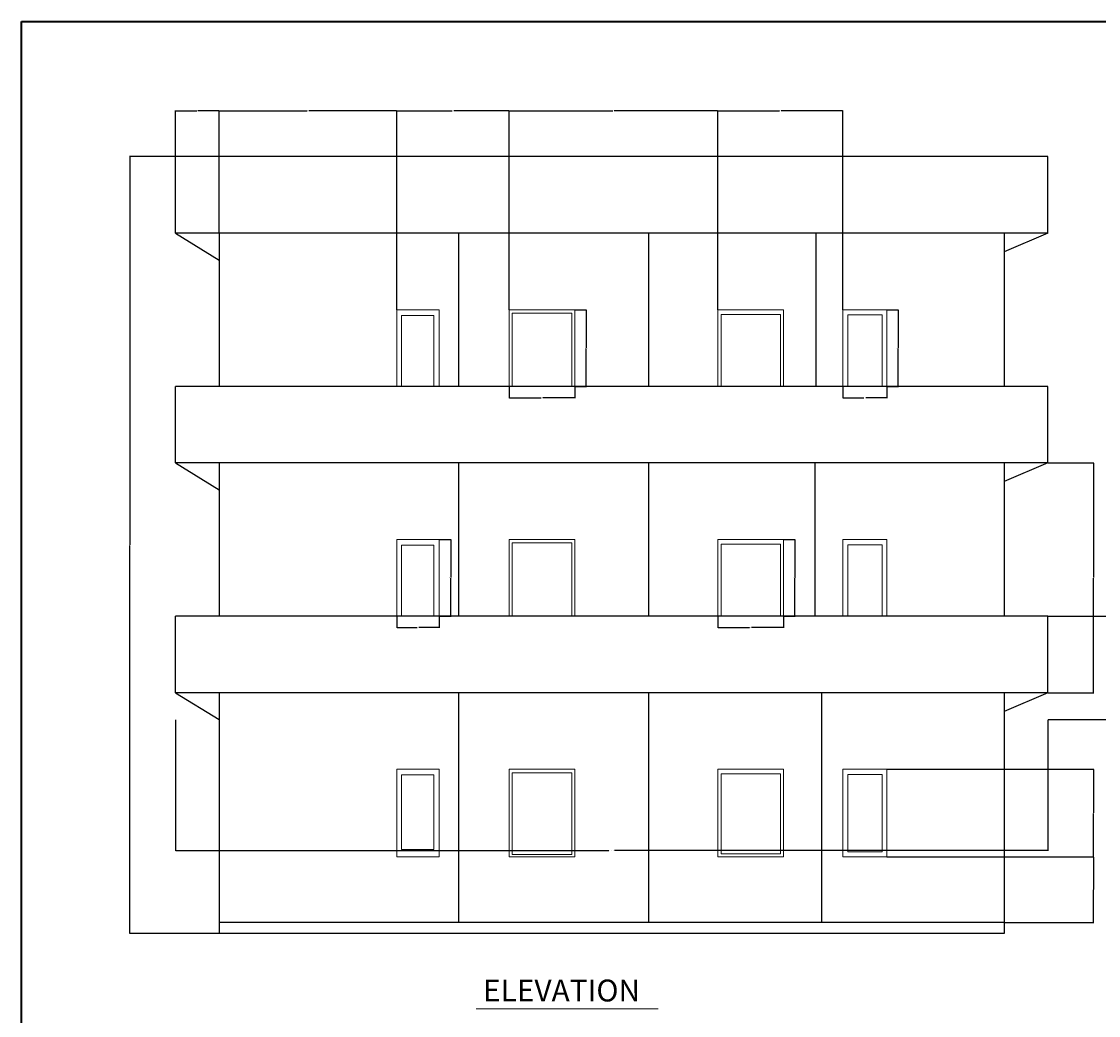
# Model space of a CAD drawing. Units: inches. Extents: x 992 to 2287, y 1476 to 2866.
# Tile 8 of 9: x 992 to 1583, y 2321 to 2866. Entities that reach past the tile are written whole.
import ezdxf

# ---------------------------------------------------------------- set-up
doc = ezdxf.new("R2010")
doc.units = ezdxf.units.IN
for name, color, linetype, lineweight in [('A-ANNO-DIMS', 2, 'Continuous', 18), ('A-ANNO-TEXT', 7, 'Continuous', 18), ('A-ANNO-TTLB', 7, 'Continuous', 35), ('A-ELEV', 7, 'Continuous', 25), ('A-GLAZ', 4, 'Continuous', 18)]:
    doc.layers.add(name, color=color, linetype=linetype, lineweight=lineweight)
doc.styles.get("Standard").update_dxf_attribs({"font": 'arial.ttf'})
doc.dimstyles.get("Standard").update_dxf_attribs({"dimtxt": 0.18, "dimasz": 0.18, "dimexe": 0.18, "dimexo": 0.0625, "dimgap": 0.09, "dimtad": 0, "dimtih": 1, "dimtoh": 1, "dimdec": 4, "dimzin": 0, "dimdsep": 46, "dimtxsty": 'Standard', "dimcen": 0.09, "dimadec": 0, "dimazin": 0, "dimtfac": 1, "dimtdec": 4, "dimtofl": 0, "dimtmove": 0, "dimatfit": 3, "dimfxl": 1, "dimtolj": 1, "dimtzin": 0, "dimarcsym": 0})

# ---------------------------------------------------------------- blocks, each defined once
blk = doc.blocks.new('WINDOW-ELEV-UPPER-A')
for p, q in [((0, 42), (0, 0)), ((23.27, 42), (0, 42)), ((0, 42), (0, 0)), ((23.27, 42), (0, 42)), ((23.27, 42), (23.27, 0)), ((23.27, 42), (23.27, 0))]:
    blk.add_line(p, q)
blk.add_lwpolyline([(2.65, 0), (2.65, 38.89), (20.39, 38.89), (20.39, 0)])
blk = doc.blocks.new('WINDOW-ELEV-UPPER-B')
for p, q in [((0, 42), (0, 0)), ((36, 42), (0, 42)), ((0, 42), (0, 0)), ((36, 42), (0, 42)), ((36, 42), (36, 0)), ((36, 42), (36, 0))]:
    blk.add_line(p, q)
blk.add_lwpolyline([(1.7, 0), (1.7, 40.14), (34.34, 40.14), (34.34, 0)])
blk = doc.blocks.new('WINDOW-ELEV-UPPER-C')
for p, q in [((0, 42), (0, 0)), ((36, 42), (0, 42)), ((0, 42), (0, 0)), ((36, 42), (0, 42)), ((36, 42), (36, 0)), ((36, 42), (36, 0))]:
    blk.add_line(p, q)
blk.add_lwpolyline([(1.97, 0), (1.97, 39.43), (34.39, 39.43), (34.39, 0)])
blk = doc.blocks.new('WINDOW-ELEV-UPPER-D')
for p, q in [((0, 42), (0, 0)), ((24, 42), (0, 42)), ((0, 42), (0, 0)), ((24, 42), (0, 42)), ((24, 42), (24, 0)), ((24, 42), (24, 0))]:
    blk.add_line(p, q)
blk.add_lwpolyline([(2.66, 0), (2.66, 39.18), (21.56, 39.18), (21.56, 0)])
blk = doc.blocks.new('PARAPET-BAND-ELEV')
for p, q in [((478.5, 56.73), (0, 56.73)), ((0, 14.73), (0, 56.73)), ((478.5, 14.73), (478.5, 56.73)), ((478.5, 14.73), (0, 14.73)), ((0, 14.73), (24, 0)), ((478.5, 14.73), (454.5, 4.48))]:
    blk.add_line(p, q)
blk = doc.blocks.new('*D93')
at = {"layer": 'A-ANNO-DIMS', "color": 0, "lineweight": -2, "transparency": 16777216}
for p, q in [((1076.79, 2483.33), (1076.79, 2411.44)), ((1555.29, 2483.33), (1555.29, 2411.44)), ((1076.97, 2411.62), (1314.44, 2411.62)), ((1555.11, 2411.62), (1317.64, 2411.62))]:
    blk.add_line(p, q, dxfattribs=at)
at = {"layer": 'A-ANNO-DIMS', "color": 0, "transparency": 16777216}
for points in [[(1076.97, 2411.65), (1076.97, 2411.59), (1076.79, 2411.62)], [(1555.11, 2411.65), (1555.11, 2411.59), (1555.29, 2411.62)]]:
    blk.add_solid(points, dxfattribs=at)
at = {"layer": 'Defpoints', "color": 0, "transparency": 16777216}
for p in [(1076.79, 2483.4), (1555.29, 2483.4), (1555.29, 2411.62)]:
    blk.add_point(p, dxfattribs=at)
at = {"layer": 'A-ANNO-DIMS', "color": 0, "transparency": 16777216, "insert": (1316.04, 2411.62), "char_height": 0.18, "attachment_point": 5}
blk.add_mtext('\\A1;PARAPET BAND 479 TYP.', dxfattribs=at)
blk = doc.blocks.new('*D94')
at = {"layer": 'A-ANNO-DIMS', "color": 0, "lineweight": -2, "transparency": 16777216}
for p, q in [((1555.36, 2540.13), (1627.25, 2540.13)), ((1627.07, 2539.95), (1627.07, 2511.94)), ((1627.07, 2483.58), (1627.07, 2511.58)), ((1555.36, 2483.4), (1627.25, 2483.4))]:
    blk.add_line(p, q, dxfattribs=at)
at = {"layer": 'A-ANNO-DIMS', "color": 0, "transparency": 16777216}
for points in [[(1627.04, 2539.95), (1627.1, 2539.95), (1627.07, 2540.13)], [(1627.04, 2483.58), (1627.1, 2483.58), (1627.07, 2483.4)]]:
    blk.add_solid(points, dxfattribs=at)
at = {"layer": 'Defpoints', "color": 0, "transparency": 16777216}
for p in [(1555.29, 2540.13), (1627.07, 2540.13), (1555.29, 2483.4)]:
    blk.add_point(p, dxfattribs=at)
at = {"layer": 'A-ANNO-DIMS', "color": 0, "transparency": 16777216, "insert": (1627.07, 2511.76), "char_height": 0.18, "attachment_point": 5}
blk.add_mtext('\\A1;57 TYP.', dxfattribs=at)
blk = doc.blocks.new('*D95')
at = {"layer": 'A-ANNO-DIMS', "color": 0, "lineweight": -2, "transparency": 16777216}
for p, q in [((1221.48, 2582.13), (1227.9, 2582.13)), ((1227.72, 2581.95), (1227.72, 2561.31)), ((1227.72, 2540.31), (1227.72, 2560.95)), ((1221.48, 2540.13), (1227.9, 2540.13))]:
    blk.add_line(p, q, dxfattribs=at)
at = {"layer": 'A-ANNO-DIMS', "color": 0, "transparency": 16777216}
for points in [[(1227.69, 2581.95), (1227.75, 2581.95), (1227.72, 2582.13)], [(1227.69, 2540.31), (1227.75, 2540.31), (1227.72, 2540.13)]]:
    blk.add_solid(points, dxfattribs=at)
at = {"layer": 'Defpoints', "color": 0, "transparency": 16777216}
for p in [(1221.42, 2582.13), (1227.72, 2582.13), (1221.42, 2540.13)]:
    blk.add_point(p, dxfattribs=at)
at = {"layer": 'A-ANNO-DIMS', "color": 0, "transparency": 16777216, "insert": (1227.72, 2561.13), "char_height": 0.18, "attachment_point": 5}
blk.add_mtext('\\A1;WIN A 42 TYP.', dxfattribs=at)
blk = doc.blocks.new('*D96')
at = {"layer": 'A-ANNO-DIMS', "color": 0, "lineweight": -2, "transparency": 16777216}
for p, q in [((1198.15, 2540.07), (1198.15, 2533.65)), ((1221.42, 2540.07), (1221.42, 2533.65)), ((1198.33, 2533.83), (1209.26, 2533.83)), ((1221.24, 2533.83), (1210.32, 2533.83))]:
    blk.add_line(p, q, dxfattribs=at)
at = {"layer": 'A-ANNO-DIMS', "color": 0, "transparency": 16777216}
for points in [[(1198.33, 2533.86), (1198.33, 2533.8), (1198.15, 2533.83)], [(1221.24, 2533.86), (1221.24, 2533.8), (1221.42, 2533.83)]]:
    blk.add_solid(points, dxfattribs=at)
at = {"layer": 'Defpoints', "color": 0, "transparency": 16777216}
for p in [(1198.15, 2540.13), (1221.42, 2540.13), (1221.42, 2533.83)]:
    blk.add_point(p, dxfattribs=at)
at = {"layer": 'A-ANNO-DIMS', "color": 0, "transparency": 16777216, "insert": (1209.79, 2533.83), "char_height": 0.18, "attachment_point": 5}
blk.add_mtext('\\A1;23 TYP.', dxfattribs=at)
blk = doc.blocks.new('*D97')
at = {"layer": 'A-ANNO-DIMS', "color": 0, "lineweight": -2, "transparency": 16777216}
for p, q in [((1295.87, 2708.13), (1302.28, 2708.13)), ((1302.1, 2707.95), (1302.1, 2687.31)), ((1302.1, 2666.31), (1302.1, 2686.95)), ((1295.87, 2666.13), (1302.28, 2666.13))]:
    blk.add_line(p, q, dxfattribs=at)
at = {"layer": 'A-ANNO-DIMS', "color": 0, "transparency": 16777216}
for points in [[(1302.07, 2707.95), (1302.13, 2707.95), (1302.1, 2708.13)], [(1302.07, 2666.31), (1302.13, 2666.31), (1302.1, 2666.13)]]:
    blk.add_solid(points, dxfattribs=at)
at = {"layer": 'Defpoints', "color": 0, "transparency": 16777216}
for p in [(1295.8, 2708.13), (1302.1, 2708.13), (1295.8, 2666.13)]:
    blk.add_point(p, dxfattribs=at)
at = {"layer": 'A-ANNO-DIMS', "color": 0, "transparency": 16777216, "insert": (1302.1, 2687.13), "char_height": 0.18, "attachment_point": 5}
blk.add_mtext('\\A1;WIN B 42 TYP.', dxfattribs=at)
blk = doc.blocks.new('*D98')
at = {"layer": 'A-ANNO-DIMS', "color": 0, "lineweight": -2, "transparency": 16777216}
for p, q in [((1259.8, 2666.07), (1259.8, 2659.65)), ((1295.8, 2666.07), (1295.8, 2659.65)), ((1259.98, 2659.83), (1277.27, 2659.83)), ((1295.62, 2659.83), (1278.33, 2659.83))]:
    blk.add_line(p, q, dxfattribs=at)
at = {"layer": 'A-ANNO-DIMS', "color": 0, "transparency": 16777216}
for points in [[(1259.98, 2659.86), (1259.98, 2659.8), (1259.8, 2659.83)], [(1295.62, 2659.86), (1295.62, 2659.8), (1295.8, 2659.83)]]:
    blk.add_solid(points, dxfattribs=at)
at = {"layer": 'Defpoints', "color": 0, "transparency": 16777216}
for p in [(1259.8, 2666.13), (1295.8, 2666.13), (1295.8, 2659.83)]:
    blk.add_point(p, dxfattribs=at)
at = {"layer": 'A-ANNO-DIMS', "color": 0, "transparency": 16777216, "insert": (1277.8, 2659.83), "char_height": 0.18, "attachment_point": 5}
blk.add_mtext('\\A1;36 TYP.', dxfattribs=at)
blk = doc.blocks.new('*D99')
at = {"layer": 'A-ANNO-DIMS', "color": 0, "lineweight": -2, "transparency": 16777216}
for p, q in [((1410.26, 2582.13), (1416.67, 2582.13)), ((1416.49, 2581.95), (1416.49, 2561.31)), ((1416.49, 2540.31), (1416.49, 2560.95)), ((1410.26, 2540.13), (1416.67, 2540.13))]:
    blk.add_line(p, q, dxfattribs=at)
at = {"layer": 'A-ANNO-DIMS', "color": 0, "transparency": 16777216}
for points in [[(1416.46, 2581.95), (1416.52, 2581.95), (1416.49, 2582.13)], [(1416.46, 2540.31), (1416.52, 2540.31), (1416.49, 2540.13)]]:
    blk.add_solid(points, dxfattribs=at)
at = {"layer": 'Defpoints', "color": 0, "transparency": 16777216}
for p in [(1410.19, 2582.13), (1416.49, 2582.13), (1410.19, 2540.13)]:
    blk.add_point(p, dxfattribs=at)
at = {"layer": 'A-ANNO-DIMS', "color": 0, "transparency": 16777216, "insert": (1416.49, 2561.13), "char_height": 0.18, "attachment_point": 5}
blk.add_mtext('\\A1;WIN C 42 TYP.', dxfattribs=at)
blk = doc.blocks.new('*D100')
at = {"layer": 'A-ANNO-DIMS', "color": 0, "lineweight": -2, "transparency": 16777216}
for p, q in [((1374.19, 2540.07), (1374.19, 2533.65)), ((1410.19, 2540.07), (1410.19, 2533.65)), ((1374.37, 2533.83), (1391.67, 2533.83)), ((1410.01, 2533.83), (1392.72, 2533.83))]:
    blk.add_line(p, q, dxfattribs=at)
at = {"layer": 'A-ANNO-DIMS', "color": 0, "transparency": 16777216}
for points in [[(1374.37, 2533.86), (1374.37, 2533.8), (1374.19, 2533.83)], [(1410.01, 2533.86), (1410.01, 2533.8), (1410.19, 2533.83)]]:
    blk.add_solid(points, dxfattribs=at)
at = {"layer": 'Defpoints', "color": 0, "transparency": 16777216}
for p in [(1374.19, 2540.13), (1410.19, 2540.13), (1410.19, 2533.83)]:
    blk.add_point(p, dxfattribs=at)
at = {"layer": 'A-ANNO-DIMS', "color": 0, "transparency": 16777216, "insert": (1392.19, 2533.83), "char_height": 0.18, "attachment_point": 5}
blk.add_mtext('\\A1;36 TYP.', dxfattribs=at)
blk = doc.blocks.new('*D101')
at = {"layer": 'A-ANNO-DIMS', "color": 0, "lineweight": -2, "transparency": 16777216}
for p, q in [((1466.92, 2708.13), (1473.34, 2708.13)), ((1473.16, 2707.95), (1473.16, 2687.31)), ((1473.16, 2666.31), (1473.16, 2686.95)), ((1466.92, 2666.13), (1473.34, 2666.13))]:
    blk.add_line(p, q, dxfattribs=at)
at = {"layer": 'A-ANNO-DIMS', "color": 0, "transparency": 16777216}
for points in [[(1473.13, 2707.95), (1473.19, 2707.95), (1473.16, 2708.13)], [(1473.13, 2666.31), (1473.19, 2666.31), (1473.16, 2666.13)]]:
    blk.add_solid(points, dxfattribs=at)
at = {"layer": 'Defpoints', "color": 0, "transparency": 16777216}
for p in [(1466.86, 2708.13), (1473.16, 2708.13), (1466.86, 2666.13)]:
    blk.add_point(p, dxfattribs=at)
at = {"layer": 'A-ANNO-DIMS', "color": 0, "transparency": 16777216, "insert": (1473.16, 2687.13), "char_height": 0.18, "attachment_point": 5}
blk.add_mtext('\\A1;WIN D 42 TYP.', dxfattribs=at)
blk = doc.blocks.new('*D102')
at = {"layer": 'A-ANNO-DIMS', "color": 0, "lineweight": -2, "transparency": 16777216}
for p, q in [((1442.86, 2666.07), (1442.86, 2659.65)), ((1466.86, 2666.07), (1466.86, 2659.65)), ((1443.04, 2659.83), (1454.33, 2659.83)), ((1466.68, 2659.83), (1455.39, 2659.83))]:
    blk.add_line(p, q, dxfattribs=at)
at = {"layer": 'A-ANNO-DIMS', "color": 0, "transparency": 16777216}
for points in [[(1443.04, 2659.86), (1443.04, 2659.8), (1442.86, 2659.83)], [(1466.68, 2659.86), (1466.68, 2659.8), (1466.86, 2659.83)]]:
    blk.add_solid(points, dxfattribs=at)
at = {"layer": 'Defpoints', "color": 0, "transparency": 16777216}
for p in [(1442.86, 2666.13), (1466.86, 2666.13), (1466.86, 2659.83)]:
    blk.add_point(p, dxfattribs=at)
at = {"layer": 'A-ANNO-DIMS', "color": 0, "transparency": 16777216, "insert": (1454.86, 2659.83), "char_height": 0.18, "attachment_point": 5}
blk.add_mtext('\\A1;24 TYP.', dxfattribs=at)
blk = doc.blocks.new('*D132')
at = {"layer": 'A-ANNO-DIMS', "color": 0, "lineweight": -2, "transparency": 16777216}
for p, q in [((1076.73, 2792.13), (1051.56, 2792.13)), ((1051.74, 2791.95), (1051.74, 2579.31)), ((1051.74, 2366.31), (1051.74, 2578.95)), ((1100.73, 2366.13), (1051.56, 2366.13))]:
    blk.add_line(p, q, dxfattribs=at)
at = {"layer": 'A-ANNO-DIMS', "color": 0, "transparency": 16777216}
for points in [[(1051.71, 2791.95), (1051.77, 2791.95), (1051.74, 2792.13)], [(1051.71, 2366.31), (1051.77, 2366.31), (1051.74, 2366.13)]]:
    blk.add_solid(points, dxfattribs=at)
at = {"layer": 'Defpoints', "color": 0, "transparency": 16777216}
for p in [(1051.74, 2792.13), (1076.79, 2792.13), (1100.79, 2366.13)]:
    blk.add_point(p, dxfattribs=at)
at = {"layer": 'A-ANNO-DIMS', "color": 0, "transparency": 16777216, "insert": (1051.74, 2579.13), "char_height": 0.18, "attachment_point": 5}
blk.add_mtext('\\A1;426', dxfattribs=at)
blk = doc.blocks.new('*D133')
at = {"layer": 'A-ANNO-DIMS', "color": 0, "lineweight": -2, "transparency": 16777216}
for p, q in [((1076.79, 2792.19), (1076.79, 2817.36)), ((1076.97, 2817.18), (1088.57, 2817.18)), ((1100.61, 2817.18), (1089.01, 2817.18)), ((1100.79, 2750.19), (1100.79, 2817.36))]:
    blk.add_line(p, q, dxfattribs=at)
at = {"layer": 'A-ANNO-DIMS', "color": 0, "transparency": 16777216}
for points in [[(1076.97, 2817.21), (1076.97, 2817.15), (1076.79, 2817.18)], [(1100.61, 2817.21), (1100.61, 2817.15), (1100.79, 2817.18)]]:
    blk.add_solid(points, dxfattribs=at)
at = {"layer": 'Defpoints', "color": 0, "transparency": 16777216}
for p in [(1100.79, 2817.18), (1076.79, 2792.13), (1100.79, 2750.13)]:
    blk.add_point(p, dxfattribs=at)
at = {"layer": 'A-ANNO-DIMS', "color": 0, "transparency": 16777216, "insert": (1088.79, 2817.18), "char_height": 0.18, "attachment_point": 5}
blk.add_mtext('\\A1;24', dxfattribs=at)
blk = doc.blocks.new('*D134')
at = {"layer": 'A-ANNO-DIMS', "color": 0, "lineweight": -2, "transparency": 16777216}
for p, q in [((1100.79, 2750.19), (1100.79, 2817.36)), ((1100.97, 2817.18), (1149.08, 2817.18)), ((1197.97, 2817.18), (1149.87, 2817.18)), ((1198.15, 2708.19), (1198.15, 2817.36))]:
    blk.add_line(p, q, dxfattribs=at)
at = {"layer": 'A-ANNO-DIMS', "color": 0, "transparency": 16777216}
for points in [[(1100.97, 2817.21), (1100.97, 2817.15), (1100.79, 2817.18)], [(1197.97, 2817.21), (1197.97, 2817.15), (1198.15, 2817.18)]]:
    blk.add_solid(points, dxfattribs=at)
at = {"layer": 'Defpoints', "color": 0, "transparency": 16777216}
for p in [(1198.15, 2817.18), (1100.79, 2750.13), (1198.15, 2708.13)]:
    blk.add_point(p, dxfattribs=at)
at = {"layer": 'A-ANNO-DIMS', "color": 0, "transparency": 16777216, "insert": (1149.47, 2817.18), "char_height": 0.18, "attachment_point": 5}
blk.add_mtext('\\A1;97.36', dxfattribs=at)
blk = doc.blocks.new('*D135')
at = {"layer": 'A-ANNO-DIMS', "color": 0, "lineweight": -2, "transparency": 16777216}
for p, q in [((1198.15, 2708.19), (1198.15, 2817.36)), ((1198.33, 2817.18), (1228.58, 2817.18)), ((1259.62, 2817.18), (1229.37, 2817.18)), ((1259.8, 2708.19), (1259.8, 2817.36))]:
    blk.add_line(p, q, dxfattribs=at)
at = {"layer": 'A-ANNO-DIMS', "color": 0, "transparency": 16777216}
for points in [[(1198.33, 2817.21), (1198.33, 2817.15), (1198.15, 2817.18)], [(1259.62, 2817.21), (1259.62, 2817.15), (1259.8, 2817.18)]]:
    blk.add_solid(points, dxfattribs=at)
at = {"layer": 'Defpoints', "color": 0, "transparency": 16777216}
for p in [(1259.8, 2817.18), (1198.15, 2708.13), (1259.8, 2708.13)]:
    blk.add_point(p, dxfattribs=at)
at = {"layer": 'A-ANNO-DIMS', "color": 0, "transparency": 16777216, "insert": (1228.98, 2817.18), "char_height": 0.18, "attachment_point": 5}
blk.add_mtext('\\A1;61.65', dxfattribs=at)
blk = doc.blocks.new('*D136')
at = {"layer": 'A-ANNO-DIMS', "color": 0, "lineweight": -2, "transparency": 16777216}
for p, q in [((1259.8, 2708.19), (1259.8, 2817.36)), ((1259.98, 2817.18), (1316.61, 2817.18)), ((1374.01, 2817.18), (1317.38, 2817.18)), ((1374.19, 2708.19), (1374.19, 2817.36))]:
    blk.add_line(p, q, dxfattribs=at)
at = {"layer": 'A-ANNO-DIMS', "color": 0, "transparency": 16777216}
for points in [[(1259.98, 2817.21), (1259.98, 2817.15), (1259.8, 2817.18)], [(1374.01, 2817.21), (1374.01, 2817.15), (1374.19, 2817.18)]]:
    blk.add_solid(points, dxfattribs=at)
at = {"layer": 'Defpoints', "color": 0, "transparency": 16777216}
for p in [(1374.19, 2817.18), (1259.8, 2708.13), (1374.19, 2708.13)]:
    blk.add_point(p, dxfattribs=at)
at = {"layer": 'A-ANNO-DIMS', "color": 0, "transparency": 16777216, "insert": (1317, 2817.18), "char_height": 0.18, "attachment_point": 5}
blk.add_mtext('\\A1;114.4', dxfattribs=at)
blk = doc.blocks.new('*D137')
at = {"layer": 'A-ANNO-DIMS', "color": 0, "lineweight": -2, "transparency": 16777216}
for p, q in [((1374.19, 2708.19), (1374.19, 2817.36)), ((1374.37, 2817.18), (1408.13, 2817.18)), ((1442.68, 2817.18), (1408.92, 2817.18)), ((1442.86, 2708.19), (1442.86, 2817.36))]:
    blk.add_line(p, q, dxfattribs=at)
at = {"layer": 'A-ANNO-DIMS', "color": 0, "transparency": 16777216}
for points in [[(1374.37, 2817.21), (1374.37, 2817.15), (1374.19, 2817.18)], [(1442.68, 2817.21), (1442.68, 2817.15), (1442.86, 2817.18)]]:
    blk.add_solid(points, dxfattribs=at)
at = {"layer": 'Defpoints', "color": 0, "transparency": 16777216}
for p in [(1442.86, 2817.18), (1374.19, 2708.13), (1442.86, 2708.13)]:
    blk.add_point(p, dxfattribs=at)
at = {"layer": 'A-ANNO-DIMS', "color": 0, "transparency": 16777216, "insert": (1408.53, 2817.18), "char_height": 0.18, "attachment_point": 5}
blk.add_mtext('\\A1;68.67', dxfattribs=at)
blk = doc.blocks.new('*D138')
at = {"layer": 'A-ANNO-DIMS', "color": 0, "lineweight": -2, "transparency": 16777216}
for p, q in [((1466.92, 2408.13), (1580.52, 2408.13)), ((1580.34, 2407.95), (1580.34, 2390.31)), ((1580.34, 2372.31), (1580.34, 2389.95)), ((1531.36, 2372.13), (1580.52, 2372.13))]:
    blk.add_line(p, q, dxfattribs=at)
at = {"layer": 'A-ANNO-DIMS', "color": 0, "transparency": 16777216}
for points in [[(1580.31, 2407.95), (1580.37, 2407.95), (1580.34, 2408.13)], [(1580.31, 2372.31), (1580.37, 2372.31), (1580.34, 2372.13)]]:
    blk.add_solid(points, dxfattribs=at)
at = {"layer": 'Defpoints', "color": 0, "transparency": 16777216}
for p in [(1466.86, 2408.13), (1580.34, 2408.13), (1531.29, 2372.13)]:
    blk.add_point(p, dxfattribs=at)
at = {"layer": 'A-ANNO-DIMS', "color": 0, "transparency": 16777216, "insert": (1580.34, 2390.13), "char_height": 0.18, "attachment_point": 5}
blk.add_mtext('\\A1;36', dxfattribs=at)
blk = doc.blocks.new('*D139')
at = {"layer": 'A-ANNO-DIMS', "color": 0, "lineweight": -2, "transparency": 16777216}
for p, q in [((1466.92, 2456.13), (1580.52, 2456.13)), ((1580.34, 2455.95), (1580.34, 2432.31)), ((1580.34, 2408.31), (1580.34, 2431.95)), ((1466.92, 2408.13), (1580.52, 2408.13))]:
    blk.add_line(p, q, dxfattribs=at)
at = {"layer": 'A-ANNO-DIMS', "color": 0, "transparency": 16777216}
for points in [[(1580.31, 2455.95), (1580.37, 2455.95), (1580.34, 2456.13)], [(1580.31, 2408.31), (1580.37, 2408.31), (1580.34, 2408.13)]]:
    blk.add_solid(points, dxfattribs=at)
at = {"layer": 'Defpoints', "color": 0, "transparency": 16777216}
for p in [(1466.86, 2456.13), (1580.34, 2456.13), (1466.86, 2408.13)]:
    blk.add_point(p, dxfattribs=at)
at = {"layer": 'A-ANNO-DIMS', "color": 0, "transparency": 16777216, "insert": (1580.34, 2432.13), "char_height": 0.18, "attachment_point": 5}
blk.add_mtext('\\A1;48', dxfattribs=at)
blk = doc.blocks.new('*D140')
at = {"layer": 'A-ANNO-DIMS', "color": 0, "lineweight": -2, "transparency": 16777216}
for p, q in [((1555.36, 2624.13), (1580.52, 2624.13)), ((1580.34, 2623.95), (1580.34, 2561.31)), ((1580.34, 2498.31), (1580.34, 2560.95)), ((1555.36, 2498.13), (1580.52, 2498.13))]:
    blk.add_line(p, q, dxfattribs=at)
at = {"layer": 'A-ANNO-DIMS', "color": 0, "transparency": 16777216}
for points in [[(1580.31, 2623.95), (1580.37, 2623.95), (1580.34, 2624.13)], [(1580.31, 2498.31), (1580.37, 2498.31), (1580.34, 2498.13)]]:
    blk.add_solid(points, dxfattribs=at)
at = {"layer": 'Defpoints', "color": 0, "transparency": 16777216}
for p in [(1555.29, 2624.13), (1580.34, 2624.13), (1555.29, 2498.13)]:
    blk.add_point(p, dxfattribs=at)
at = {"layer": 'A-ANNO-DIMS', "color": 0, "transparency": 16777216, "insert": (1580.34, 2561.13), "char_height": 0.18, "attachment_point": 5}
blk.add_mtext('\\A1;126', dxfattribs=at)

msp = doc.modelspace()

# ---------------------------------------------------------------- linework, layer by layer
at = {"layer": 'A-ANNO-TEXT'}
msp.add_line((1241.7212, 2324.7684), (1341.5908, 2324.7684), dxfattribs=at)
at = {"layer": 'A-ANNO-TTLB'}
msp.add_lwpolyline([(992.3484, 2866.1952), (2287.217, 2866.1952), (2287.217, 1476.4066), (992.3484, 1476.4066)], close=True, dxfattribs=at)
at = {"layer": 'A-ELEV'}
for p, q in [((1100.7936, 2750.1302), (1100.7936, 2666.1302)), ((1232.0825, 2750.1302), (1232.0825, 2666.1302)), ((1336.2936, 2750.1302), (1336.2936, 2666.1302)), ((1428.1613, 2666.1302), (1428.1613, 2750.1302)), ((1531.2936, 2750.1302), (1531.2936, 2666.1302)), ((1100.7936, 2624.1302), (1100.7936, 2540.1302)), ((1100.7936, 2624.1302), (1100.7936, 2618.1302)), ((1232.0825, 2624.1302), (1232.0825, 2540.1302)), ((1336.2936, 2624.1302), (1336.2936, 2540.1302)), ((1427.6159, 2540.1302), (1427.6159, 2624.1302)), ((1531.2936, 2624.1302), (1531.2936, 2540.1302)), ((1531.2936, 2624.1302), (1531.2936, 2618.1302)), ((1100.7936, 2498.1302), (1100.7936, 2366.1302)), ((1100.7936, 2498.1302), (1100.7936, 2492.1302)), ((1232.0825, 2498.1302), (1232.0825, 2372.1302)), ((1336.2936, 2498.1302), (1336.2936, 2372.1302)), ((1431.3852, 2372.1302), (1431.3852, 2498.1302)), ((1531.2936, 2498.1302), (1531.2936, 2366.1302)), ((1531.2936, 2498.1302), (1531.2936, 2492.1302)), ((1531.2936, 2372.1302), (1100.7936, 2372.1302)), ((1531.2936, 2366.1302), (1100.7936, 2366.1302))]:
    msp.add_line(p, q, dxfattribs=at)
at = {"layer": 'A-GLAZ'}
for p, q in [((1198.1541, 2456.1302), (1198.1541, 2408.1302)), ((1221.421, 2456.1302), (1198.1541, 2456.1302)), ((1221.421, 2456.1302), (1221.421, 2408.1302)), ((1259.8028, 2456.1302), (1259.8028, 2408.1302)), ((1295.8028, 2456.1302), (1259.8028, 2456.1302)), ((1295.8028, 2456.1302), (1295.8028, 2408.1302)), ((1374.1932, 2456.1302), (1374.1932, 2408.1302)), ((1410.1932, 2456.1302), (1374.1932, 2456.1302)), ((1410.1932, 2456.1302), (1410.1932, 2408.1302)), ((1442.8592, 2456.1302), (1442.8592, 2408.1302)), ((1466.8592, 2456.1302), (1442.8592, 2456.1302)), ((1466.8592, 2456.1302), (1466.8592, 2408.1302)), ((1221.421, 2408.1302), (1198.1541, 2408.1302)), ((1295.8028, 2408.1302), (1259.8028, 2408.1302)), ((1410.1932, 2408.1302), (1374.1932, 2408.1302)), ((1466.8592, 2408.1302), (1442.8592, 2408.1302))]:
    msp.add_line(p, q, dxfattribs=at)
for points in [[(1200.8045, 2453.018), (1218.5431, 2453.018), (1218.5431, 2412.1782), (1200.8045, 2412.1782)], [(1261.5013, 2454.2712), (1294.1453, 2454.2712), (1294.1453, 2409.335), (1261.5013, 2409.335)], [(1376.1619, 2453.5613), (1408.5872, 2453.5613), (1408.5872, 2409.7014), (1376.1619, 2409.7014)], [(1445.5232, 2453.3126), (1464.4228, 2453.3126), (1464.4228, 2410.8364), (1445.5232, 2410.8364)]]:
    msp.add_lwpolyline(points, close=True, dxfattribs=at)

# ---------------------------------------------------------------- block references
at = {"layer": 'A-ELEV'}
for p in [(1076.794, 2735.396), (1076.794, 2609.396), (1076.794, 2483.396)]:
    msp.add_blockref('PARAPET-BAND-ELEV', p, dxfattribs=at)
at = {"layer": 'A-GLAZ'}
for name, p in [('WINDOW-ELEV-UPPER-A', (1198.154, 2666.13)), ('WINDOW-ELEV-UPPER-B', (1259.803, 2666.13)), ('WINDOW-ELEV-UPPER-C', (1374.193, 2666.13)), ('WINDOW-ELEV-UPPER-D', (1442.859, 2666.13)), ('WINDOW-ELEV-UPPER-A', (1198.154, 2540.13)), ('WINDOW-ELEV-UPPER-B', (1259.803, 2540.13)), ('WINDOW-ELEV-UPPER-C', (1374.193, 2540.13)), ('WINDOW-ELEV-UPPER-D', (1442.859, 2540.13))]:
    msp.add_blockref(name, p, dxfattribs=at)

# ---------------------------------------------------------------- texts
at = {"layer": 'A-ANNO-TEXT', "insert": (1245.4834, 2340.817), "char_height": 12, "attachment_point": 1}
msp.add_mtext_dynamic_manual_height_columns('ELEVATION', width=252.247358, gutter_width=12.5, heights=[0], dxfattribs=at)

# ---------------------------------------------------------------- dimensions: what is measured, and where the dimension line sits
at = {"layer": 'A-ANNO-DIMS'}
for base, p1, p2, override, picture, middle in [((1100.7936, 2817.1802), (1076.7936, 2792.1302), (1100.7936, 2750.1302), {"dimdec": 0, "dimlfac": 1, "dimrnd": 0, "dimzin": 0, "dimdsep": 46, "dimlunit": 2}, '*D133', (1088.7936, 2817.1802)), ((1198.1541, 2817.1802), (1100.7936, 2750.1302), (1198.1541, 2708.1302), {"dimdec": 2, "dimlfac": 1, "dimrnd": 0, "dimzin": 0, "dimdsep": 46, "dimlunit": 2}, '*D134', (1149.4738, 2817.1802)), ((1259.8028, 2817.1802), (1198.1541, 2708.1302), (1259.8028, 2708.1302), {"dimdec": 2, "dimlfac": 1, "dimrnd": 0, "dimzin": 0, "dimdsep": 46, "dimlunit": 2}, '*D135', (1228.9784, 2817.1802)), ((1374.1932, 2817.1802), (1259.8028, 2708.1302), (1374.1932, 2708.1302), {"dimdec": 1, "dimlfac": 1, "dimrnd": 0, "dimzin": 0, "dimdsep": 46, "dimlunit": 2}, '*D136', (1316.998, 2817.1802)), ((1442.8592, 2817.1802), (1374.1932, 2708.1302), (1442.8592, 2708.1302), {"dimdec": 2, "dimlfac": 1, "dimrnd": 0, "dimzin": 0, "dimdsep": 46, "dimlunit": 2}, '*D137', (1408.5262, 2817.1802))]:
    dim = msp.add_linear_dim(base=base, p1=p1, p2=p2, dimstyle='Standard', override=override, dxfattribs=at)
    dim.commit()
    dim.dimension.update_dxf_attribs({"geometry": picture, "text_midpoint": middle})
for base, p1, p2, picture, middle in [((1051.7436, 2792.1302), (1100.7936, 2366.1302), (1076.7936, 2792.1302), '*D132', (1051.7436, 2579.1302)), ((1580.3436, 2624.1302), (1555.2936, 2498.1302), (1555.2936, 2624.1302), '*D140', (1580.3436, 2561.1302)), ((1580.3436, 2456.1302), (1466.8592, 2408.1302), (1466.8592, 2456.1302), '*D139', (1580.3436, 2432.1302)), ((1580.3436, 2408.1302), (1531.2936, 2372.1302), (1466.8592, 2408.1302), '*D138', (1580.3436, 2390.1302))]:
    dim = msp.add_linear_dim(base=base, p1=p1, p2=p2, angle=90, dimstyle='Standard', override={"dimdec": 0, "dimlfac": 1, "dimrnd": 0, "dimzin": 0, "dimdsep": 46, "dimlunit": 2}, dxfattribs=at)
    dim.commit()
    dim.dimension.update_dxf_attribs({"geometry": picture, "text_midpoint": middle})
for base, p1, p2, text, picture, middle in [((1302.1028, 2708.1302), (1295.8028, 2666.1302), (1295.8028, 2708.1302), 'WIN B <> TYP.', '*D97', (1302.1028, 2687.1302)), ((1473.1592, 2708.1302), (1466.8592, 2666.1302), (1466.8592, 2708.1302), 'WIN D <> TYP.', '*D101', (1473.1592, 2687.1302)), ((1227.721, 2582.1302), (1221.421, 2540.1302), (1221.421, 2582.1302), 'WIN A <> TYP.', '*D95', (1227.721, 2561.1302)), ((1416.4932, 2582.1302), (1410.1932, 2540.1302), (1410.1932, 2582.1302), 'WIN C <> TYP.', '*D99', (1416.4932, 2561.1302)), ((1627.0686, 2540.1302), (1555.2936, 2483.396), (1555.2936, 2540.1302), '<> TYP.', '*D94', (1627.0686, 2511.7631))]:
    dim = msp.add_linear_dim(base=base, p1=p1, p2=p2, angle=90, text=text, dimstyle='Standard', override={"dimdec": 0, "dimlfac": 1, "dimrnd": 0, "dimzin": 0, "dimdsep": 46, "dimlunit": 2}, dxfattribs=at)
    dim.commit()
    dim.dimension.update_dxf_attribs({"geometry": picture, "text_midpoint": middle})
for base, p1, p2, text, picture, middle in [((1295.8028, 2659.8302), (1259.8028, 2666.1302), (1295.8028, 2666.1302), '<> TYP.', '*D98', (1277.8028, 2659.8302)), ((1466.8592, 2659.8302), (1442.8592, 2666.1302), (1466.8592, 2666.1302), '<> TYP.', '*D102', (1454.8592, 2659.8302)), ((1221.421, 2533.8302), (1198.1541, 2540.1302), (1221.421, 2540.1302), '<> TYP.', '*D96', (1209.7875, 2533.8302)), ((1410.1932, 2533.8302), (1374.1932, 2540.1302), (1410.1932, 2540.1302), '<> TYP.', '*D100', (1392.1932, 2533.8302)), ((1555.2935507769, 2411.6210344275), (1076.7935507769, 2483.3960344275), (1555.2935507769, 2483.3960344275), 'PARAPET BAND <> TYP.', '*D93', (1316.0435507769, 2411.6210344275))]:
    dim = msp.add_linear_dim(base=base, p1=p1, p2=p2, text=text, dimstyle='Standard', override={"dimdec": 0, "dimlfac": 1, "dimrnd": 0, "dimzin": 0, "dimdsep": 46, "dimlunit": 2}, dxfattribs=at)
    dim.commit()
    dim.dimension.update_dxf_attribs({"geometry": picture, "text_midpoint": middle})

doc.saveas('drawing.dxf')
